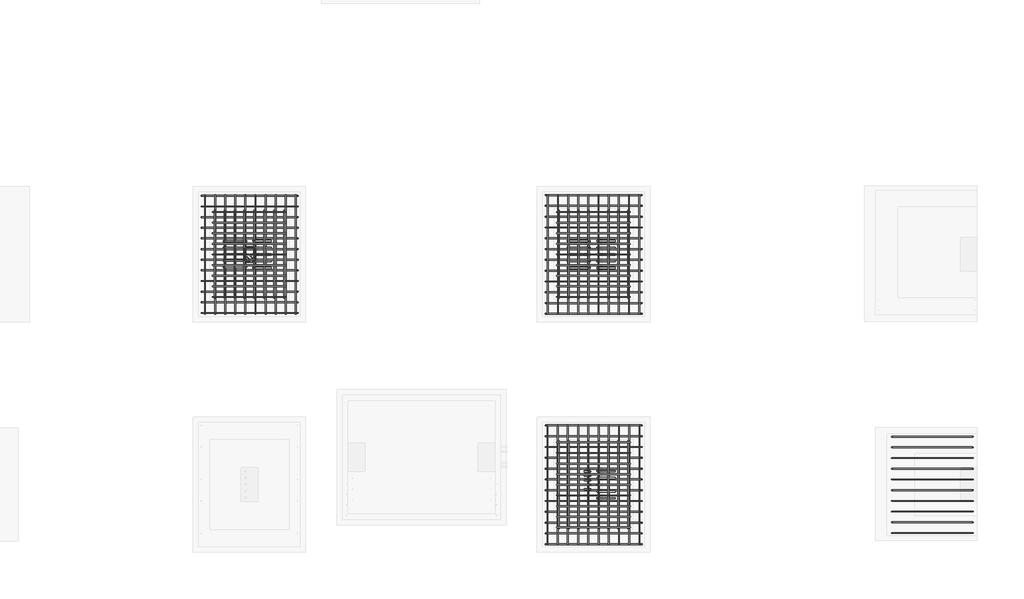
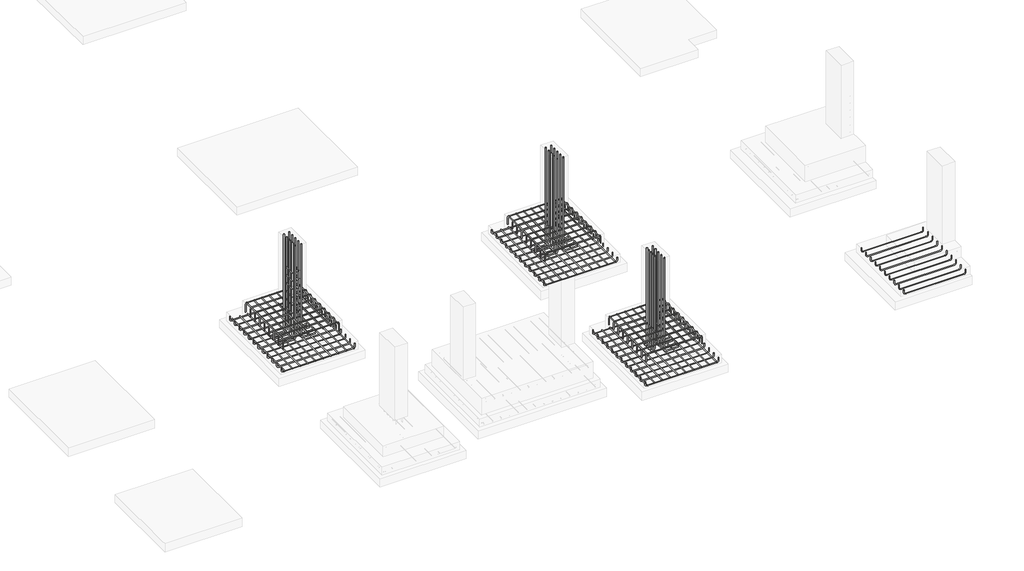
# One storey, part 4 of 6: 20 reinforcing bars.
"""IFC4 building model written with IfcOpenShell, lengths in millimetres."""

from ifc_helpers import new_model, si_unit, point, frame, origin, place, context, project, spatial, polyline, circle_curve, trimmed, segment, composite_curve, source, transform, mapped, element, save
from ifc_brep_helpers import swept_disk

model = new_model("IFC4")

# Units and contexts
model_context = context("Model", 3, world=origin())
ifc_project = project(units=[si_unit("LENGTHUNIT", "METRE", prefix="MILLI")], contexts=[model_context])

# Site, building, storey
site = spatial("IfcSite", under=ifc_project)
building = spatial("IfcBuilding", under=site)
storey = spatial("IfcBuildingStorey", under=building, Elevation=-1828.8)

# Reinforcing bars
placement = place(None, origin())
reinforcing_bar_shape = source(origin(), model_context, "Body", "SolidModel", [
    swept_disk(composite_curve([segment(polyline([(5667706.2007829, -3593857.0523052, -1806.8936208), (5667706.2007829, -3595473.4523052, -1806.8936208)]), True, "CONTINUOUS")], self_intersect=False), 6.0),
])
element("IfcReinforcingBar", 1, at=placement, inside=storey, context=model_context, shape_type="MappedRepresentation", body=[
    mapped(reinforcing_bar_shape, transform((0.0, 0.0, 0.0), x_axis=(1.0, 0.0, 0.0), y_axis=(0.0, 1.0, 0.0), z_axis=(0.0, 0.0, 1.0))),
    mapped(reinforcing_bar_shape, transform((-136.3485017, 0.0, 0.0), x_axis=(1.0, 0.0, 0.0), y_axis=(0.0, 1.0, 0.0), z_axis=(0.0, 0.0, 1.0))),
    mapped(reinforcing_bar_shape, transform((-272.6970034, 0.0, 0.0), x_axis=(1.0, 0.0, 0.0), y_axis=(0.0, 1.0, 0.0), z_axis=(0.0, 0.0, 1.0))),
    mapped(reinforcing_bar_shape, transform((-409.0455051, 0.0, 0.0), x_axis=(1.0, 0.0, 0.0), y_axis=(0.0, 1.0, 0.0), z_axis=(0.0, 0.0, 1.0))),
    mapped(reinforcing_bar_shape, transform((-545.3940068, 0.0, 0.0), x_axis=(1.0, 0.0, 0.0), y_axis=(0.0, 1.0, 0.0), z_axis=(0.0, 0.0, 1.0))),
    mapped(reinforcing_bar_shape, transform((-681.7425085, 0.0, 0.0), x_axis=(1.0, 0.0, 0.0), y_axis=(0.0, 1.0, 0.0), z_axis=(0.0, 0.0, 1.0))),
    mapped(reinforcing_bar_shape, transform((-818.0910101, 0.0, 0.0), x_axis=(1.0, 0.0, 0.0), y_axis=(0.0, 1.0, 0.0), z_axis=(0.0, 0.0, 1.0))),
    mapped(reinforcing_bar_shape, transform((-954.4395118, 0.0, 0.0), x_axis=(1.0, 0.0, 0.0), y_axis=(0.0, 1.0, 0.0), z_axis=(0.0, 0.0, 1.0))),
    mapped(reinforcing_bar_shape, transform((-1090.7880135, 0.0, 0.0), x_axis=(1.0, 0.0, 0.0), y_axis=(0.0, 1.0, 0.0), z_axis=(0.0, 0.0, 1.0))),
    mapped(reinforcing_bar_shape, transform((-1227.1365152, 0.0, 0.0), x_axis=(1.0, 0.0, 0.0), y_axis=(0.0, 1.0, 0.0), z_axis=(0.0, 0.0, 1.0))),
])
reinforcing_bar_2_shape = source(origin(), model_context, "Body", "SolidModel", [
    swept_disk(composite_curve([segment(polyline([(5666582.9165246, -3595238.8523052, -1571.6), (5666582.9165246, -3595238.8523052, -1437.6)]), True, "CONTINUOUS"), segment(trimmed(circle_curve(frame((5666612.9165246, -3595238.8523052, -1437.6), z_axis=(0.0, 1.0, 0.0), x_axis=(-30.0, 0.0, 0.0)), 30.0), [point((5666582.9165246, -3595238.8523052, -1437.6))], [point((5666612.9165246, -3595238.8523052, -1407.6))], True, "CARTESIAN"), True, "CONTINUOUS"), segment(polyline([(5666612.9165246, -3595238.8523052, -1407.6), (5667542.5447698, -3595238.8523052, -1407.6)]), True, "CONTINUOUS"), segment(trimmed(circle_curve(frame((5667542.5447698, -3595238.8523052, -1437.6), z_axis=(0.0, 1.0, 0.0), x_axis=(0.0, 0.0, 30.0)), 30.0), [point((5667542.5447698, -3595238.8523052, -1407.6))], [point((5667572.5447698, -3595238.8523052, -1437.6))], True, "CARTESIAN"), True, "CONTINUOUS"), segment(polyline([(5667572.5447698, -3595238.8523052, -1437.6), (5667572.5447698, -3595238.8523052, -1571.6)]), True, "CONTINUOUS")], self_intersect=False), 6.0),
])
element("IfcReinforcingBar", 2, at=placement, inside=storey, context=model_context, shape_type="MappedRepresentation", body=[
    mapped(reinforcing_bar_2_shape, transform((0.0, 0.0, 0.0), x_axis=(1.0, 0.0, 0.0), y_axis=(0.0, 1.0, 0.0), z_axis=(0.0, 0.0, 1.0))),
    mapped(reinforcing_bar_2_shape, transform((0.0, 143.4, 0.0), x_axis=(1.0, 0.0, 0.0), y_axis=(0.0, 1.0, 0.0), z_axis=(0.0, 0.0, 1.0))),
    mapped(reinforcing_bar_2_shape, transform((0.0, 286.8, 0.0), x_axis=(1.0, 0.0, 0.0), y_axis=(0.0, 1.0, 0.0), z_axis=(0.0, 0.0, 1.0))),
    mapped(reinforcing_bar_2_shape, transform((0.0, 430.2, 0.0), x_axis=(1.0, 0.0, 0.0), y_axis=(0.0, 1.0, 0.0), z_axis=(0.0, 0.0, 1.0))),
    mapped(reinforcing_bar_2_shape, transform((0.0, 573.6, 0.0), x_axis=(1.0, 0.0, 0.0), y_axis=(0.0, 1.0, 0.0), z_axis=(0.0, 0.0, 1.0))),
    mapped(reinforcing_bar_2_shape, transform((0.0, 717.0, 0.0), x_axis=(1.0, 0.0, 0.0), y_axis=(0.0, 1.0, 0.0), z_axis=(0.0, 0.0, 1.0))),
    mapped(reinforcing_bar_2_shape, transform((0.0, 860.4, 0.0), x_axis=(1.0, 0.0, 0.0), y_axis=(0.0, 1.0, 0.0), z_axis=(0.0, 0.0, 1.0))),
    mapped(reinforcing_bar_2_shape, transform((0.0, 1003.8, 0.0), x_axis=(1.0, 0.0, 0.0), y_axis=(0.0, 1.0, 0.0), z_axis=(0.0, 0.0, 1.0))),
    mapped(reinforcing_bar_2_shape, transform((0.0, 1147.2, 0.0), x_axis=(1.0, 0.0, 0.0), y_axis=(0.0, 1.0, 0.0), z_axis=(0.0, 0.0, 1.0))),
])
reinforcing_bar_3_shape = source(origin(), model_context, "Body", "SolidModel", [
    swept_disk(composite_curve([segment(polyline([(5666607.9580652, -3595258.3223129, -1420.5088801), (5666607.9580652, -3594070.7578875, -1420.5088801)]), True, "CONTINUOUS")], self_intersect=False), 6.0),
])
element("IfcReinforcingBar", 3, at=placement, inside=storey, context=model_context, shape_type="MappedRepresentation", body=[
    mapped(reinforcing_bar_3_shape, transform((0.0, 0.0, 0.0), x_axis=(1.0, 0.0, 0.0), y_axis=(0.0, 1.0, 0.0), z_axis=(0.0, 0.0, 1.0))),
    mapped(reinforcing_bar_3_shape, transform((134.2057348, 0.0, 0.0), x_axis=(1.0, 0.0, 0.0), y_axis=(0.0, 1.0, 0.0), z_axis=(0.0, 0.0, 1.0))),
    mapped(reinforcing_bar_3_shape, transform((268.4114695, 0.0, 0.0), x_axis=(1.0, 0.0, 0.0), y_axis=(0.0, 1.0, 0.0), z_axis=(0.0, 0.0, 1.0))),
    mapped(reinforcing_bar_3_shape, transform((402.6172043, 0.0, 0.0), x_axis=(1.0, 0.0, 0.0), y_axis=(0.0, 1.0, 0.0), z_axis=(0.0, 0.0, 1.0))),
    mapped(reinforcing_bar_3_shape, transform((536.8229391, 0.0, 0.0), x_axis=(1.0, 0.0, 0.0), y_axis=(0.0, 1.0, 0.0), z_axis=(0.0, 0.0, 1.0))),
    mapped(reinforcing_bar_3_shape, transform((671.0286738, 0.0, 0.0), x_axis=(1.0, 0.0, 0.0), y_axis=(0.0, 1.0, 0.0), z_axis=(0.0, 0.0, 1.0))),
    mapped(reinforcing_bar_3_shape, transform((805.2344086, 0.0, 0.0), x_axis=(1.0, 0.0, 0.0), y_axis=(0.0, 1.0, 0.0), z_axis=(0.0, 0.0, 1.0))),
    mapped(reinforcing_bar_3_shape, transform((939.4401433, 0.0, 0.0), x_axis=(1.0, 0.0, 0.0), y_axis=(0.0, 1.0, 0.0), z_axis=(0.0, 0.0, 1.0))),
])
reinforcing_bar_4_shape = source(origin(), model_context, "Body", "SolidModel", [
    swept_disk(composite_curve([segment(polyline([(5672341.0341193, -3593857.0523052, -1804.5123708), (5672341.0341193, -3595473.4523052, -1804.5123708)]), True, "CONTINUOUS")], self_intersect=False), 6.0),
])
element("IfcReinforcingBar", 4, at=placement, inside=storey, context=model_context, shape_type="MappedRepresentation", body=[
    mapped(reinforcing_bar_4_shape, transform((0.0, 0.0, 0.0), x_axis=(1.0, 0.0, 0.0), y_axis=(0.0, 1.0, 0.0), z_axis=(0.0, 0.0, 1.0))),
    mapped(reinforcing_bar_4_shape, transform((-136.9779353, 0.0, 0.0), x_axis=(1.0, 0.0, 0.0), y_axis=(0.0, 1.0, 0.0), z_axis=(0.0, 0.0, 1.0))),
    mapped(reinforcing_bar_4_shape, transform((-273.9558706, 0.0, 0.0), x_axis=(1.0, 0.0, 0.0), y_axis=(0.0, 1.0, 0.0), z_axis=(0.0, 0.0, 1.0))),
    mapped(reinforcing_bar_4_shape, transform((-410.9338059, 0.0, 0.0), x_axis=(1.0, 0.0, 0.0), y_axis=(0.0, 1.0, 0.0), z_axis=(0.0, 0.0, 1.0))),
    mapped(reinforcing_bar_4_shape, transform((-547.9117413, 0.0, 0.0), x_axis=(1.0, 0.0, 0.0), y_axis=(0.0, 1.0, 0.0), z_axis=(0.0, 0.0, 1.0))),
    mapped(reinforcing_bar_4_shape, transform((-684.8896766, 0.0, 0.0), x_axis=(1.0, 0.0, 0.0), y_axis=(0.0, 1.0, 0.0), z_axis=(0.0, 0.0, 1.0))),
    mapped(reinforcing_bar_4_shape, transform((-821.8676119, 0.0, 0.0), x_axis=(1.0, 0.0, 0.0), y_axis=(0.0, 1.0, 0.0), z_axis=(0.0, 0.0, 1.0))),
    mapped(reinforcing_bar_4_shape, transform((-958.8455472, 0.0, 0.0), x_axis=(1.0, 0.0, 0.0), y_axis=(0.0, 1.0, 0.0), z_axis=(0.0, 0.0, 1.0))),
    mapped(reinforcing_bar_4_shape, transform((-1095.8234825, 0.0, 0.0), x_axis=(1.0, 0.0, 0.0), y_axis=(0.0, 1.0, 0.0), z_axis=(0.0, 0.0, 1.0))),
    mapped(reinforcing_bar_4_shape, transform((-1232.8014178, 0.0, 0.0), x_axis=(1.0, 0.0, 0.0), y_axis=(0.0, 1.0, 0.0), z_axis=(0.0, 0.0, 1.0))),
])
reinforcing_bar_5_shape = source(origin(), model_context, "Body", "SolidModel", [
    swept_disk(composite_curve([segment(polyline([(5671231.1165246, -3595238.8523052, -1551.6), (5671231.1165246, -3595238.8523052, -1437.6)]), True, "CONTINUOUS"), segment(trimmed(circle_curve(frame((5671261.1165246, -3595238.8523052, -1437.6), z_axis=(0.0, 1.0, 0.0), x_axis=(-30.0, 0.0, 0.0)), 30.0), [point((5671231.1165246, -3595238.8523052, -1437.6))], [point((5671261.1165246, -3595238.8523052, -1407.6))], True, "CARTESIAN"), True, "CONTINUOUS"), segment(polyline([(5671261.1165246, -3595238.8523052, -1407.6), (5672186.288821, -3595238.8523052, -1407.6)]), True, "CONTINUOUS"), segment(trimmed(circle_curve(frame((5672186.288821, -3595238.8523052, -1437.6), z_axis=(0.0, 1.0, 0.0), x_axis=(0.0, 0.0, 30.0)), 30.0), [point((5672186.288821, -3595238.8523052, -1407.6))], [point((5672216.288821, -3595238.8523052, -1437.6))], True, "CARTESIAN"), True, "CONTINUOUS"), segment(polyline([(5672216.288821, -3595238.8523052, -1437.6), (5672216.288821, -3595238.8523052, -1551.6)]), True, "CONTINUOUS")], self_intersect=False), 6.0),
])
element("IfcReinforcingBar", 5, at=placement, inside=storey, context=model_context, shape_type="MappedRepresentation", body=[
    mapped(reinforcing_bar_5_shape, transform((0.0, 0.0, 0.0), x_axis=(1.0, 0.0, 0.0), y_axis=(0.0, 1.0, 0.0), z_axis=(0.0, 0.0, 1.0))),
    mapped(reinforcing_bar_5_shape, transform((0.0, 143.4, 0.0), x_axis=(1.0, 0.0, 0.0), y_axis=(0.0, 1.0, 0.0), z_axis=(0.0, 0.0, 1.0))),
    mapped(reinforcing_bar_5_shape, transform((0.0, 286.8, 0.0), x_axis=(1.0, 0.0, 0.0), y_axis=(0.0, 1.0, 0.0), z_axis=(0.0, 0.0, 1.0))),
    mapped(reinforcing_bar_5_shape, transform((0.0, 430.2, 0.0), x_axis=(1.0, 0.0, 0.0), y_axis=(0.0, 1.0, 0.0), z_axis=(0.0, 0.0, 1.0))),
    mapped(reinforcing_bar_5_shape, transform((0.0, 573.6, 0.0), x_axis=(1.0, 0.0, 0.0), y_axis=(0.0, 1.0, 0.0), z_axis=(0.0, 0.0, 1.0))),
    mapped(reinforcing_bar_5_shape, transform((0.0, 717.0, 0.0), x_axis=(1.0, 0.0, 0.0), y_axis=(0.0, 1.0, 0.0), z_axis=(0.0, 0.0, 1.0))),
    mapped(reinforcing_bar_5_shape, transform((0.0, 860.4, 0.0), x_axis=(1.0, 0.0, 0.0), y_axis=(0.0, 1.0, 0.0), z_axis=(0.0, 0.0, 1.0))),
    mapped(reinforcing_bar_5_shape, transform((0.0, 1003.8, 0.0), x_axis=(1.0, 0.0, 0.0), y_axis=(0.0, 1.0, 0.0), z_axis=(0.0, 0.0, 1.0))),
    mapped(reinforcing_bar_5_shape, transform((0.0, 1147.2, 0.0), x_axis=(1.0, 0.0, 0.0), y_axis=(0.0, 1.0, 0.0), z_axis=(0.0, 0.0, 1.0))),
])
reinforcing_bar_6_shape = source(origin(), model_context, "Body", "SolidModel", [
    swept_disk(composite_curve([segment(polyline([(5671259.1917143, -3595258.3223129, -1419.7151301), (5671259.1917143, -3594070.7578875, -1419.7151301)]), True, "CONTINUOUS")], self_intersect=False), 6.0),
])
element("IfcReinforcingBar", 6, at=placement, inside=storey, context=model_context, shape_type="MappedRepresentation", body=[
    mapped(reinforcing_bar_6_shape, transform((0.0, 0.0, 0.0), x_axis=(1.0, 0.0, 0.0), y_axis=(0.0, 1.0, 0.0), z_axis=(0.0, 0.0, 1.0))),
    mapped(reinforcing_bar_6_shape, transform((133.142035, 0.0, 0.0), x_axis=(1.0, 0.0, 0.0), y_axis=(0.0, 1.0, 0.0), z_axis=(0.0, 0.0, 1.0))),
    mapped(reinforcing_bar_6_shape, transform((266.28407, 0.0, 0.0), x_axis=(1.0, 0.0, 0.0), y_axis=(0.0, 1.0, 0.0), z_axis=(0.0, 0.0, 1.0))),
    mapped(reinforcing_bar_6_shape, transform((399.426105, 0.0, 0.0), x_axis=(1.0, 0.0, 0.0), y_axis=(0.0, 1.0, 0.0), z_axis=(0.0, 0.0, 1.0))),
    mapped(reinforcing_bar_6_shape, transform((532.56814, 0.0, 0.0), x_axis=(1.0, 0.0, 0.0), y_axis=(0.0, 1.0, 0.0), z_axis=(0.0, 0.0, 1.0))),
    mapped(reinforcing_bar_6_shape, transform((665.7101749, 0.0, 0.0), x_axis=(1.0, 0.0, 0.0), y_axis=(0.0, 1.0, 0.0), z_axis=(0.0, 0.0, 1.0))),
    mapped(reinforcing_bar_6_shape, transform((798.8522099, 0.0, 0.0), x_axis=(1.0, 0.0, 0.0), y_axis=(0.0, 1.0, 0.0), z_axis=(0.0, 0.0, 1.0))),
    mapped(reinforcing_bar_6_shape, transform((931.9942449, 0.0, 0.0), x_axis=(1.0, 0.0, 0.0), y_axis=(0.0, 1.0, 0.0), z_axis=(0.0, 0.0, 1.0))),
])
reinforcing_bar_7_shape = source(origin(), model_context, "Body", "SolidModel", [
    swept_disk(composite_curve([segment(polyline([(5672346.3995476, -3596967.8875145, -1801.3373708), (5672346.3995476, -3598584.2875145, -1801.3373708)]), True, "CONTINUOUS")], self_intersect=False), 6.0),
])
element("IfcReinforcingBar", 7, at=placement, inside=storey, context=model_context, shape_type="MappedRepresentation", body=[
    mapped(reinforcing_bar_7_shape, transform((0.0, 0.0, 0.0), x_axis=(1.0, 0.0, 0.0), y_axis=(0.0, 1.0, 0.0), z_axis=(0.0, 0.0, 1.0))),
    mapped(reinforcing_bar_7_shape, transform((-138.145428, 0.0, 0.0), x_axis=(1.0, 0.0, 0.0), y_axis=(0.0, 1.0, 0.0), z_axis=(0.0, 0.0, 1.0))),
    mapped(reinforcing_bar_7_shape, transform((-276.2908559, 0.0, 0.0), x_axis=(1.0, 0.0, 0.0), y_axis=(0.0, 1.0, 0.0), z_axis=(0.0, 0.0, 1.0))),
    mapped(reinforcing_bar_7_shape, transform((-414.4362839, 0.0, 0.0), x_axis=(1.0, 0.0, 0.0), y_axis=(0.0, 1.0, 0.0), z_axis=(0.0, 0.0, 1.0))),
    mapped(reinforcing_bar_7_shape, transform((-552.5817118, 0.0, 0.0), x_axis=(1.0, 0.0, 0.0), y_axis=(0.0, 1.0, 0.0), z_axis=(0.0, 0.0, 1.0))),
    mapped(reinforcing_bar_7_shape, transform((-690.7271398, 0.0, 0.0), x_axis=(1.0, 0.0, 0.0), y_axis=(0.0, 1.0, 0.0), z_axis=(0.0, 0.0, 1.0))),
    mapped(reinforcing_bar_7_shape, transform((-828.8725677, 0.0, 0.0), x_axis=(1.0, 0.0, 0.0), y_axis=(0.0, 1.0, 0.0), z_axis=(0.0, 0.0, 1.0))),
    mapped(reinforcing_bar_7_shape, transform((-967.0179957, 0.0, 0.0), x_axis=(1.0, 0.0, 0.0), y_axis=(0.0, 1.0, 0.0), z_axis=(0.0, 0.0, 1.0))),
    mapped(reinforcing_bar_7_shape, transform((-1105.1634236, 0.0, 0.0), x_axis=(1.0, 0.0, 0.0), y_axis=(0.0, 1.0, 0.0), z_axis=(0.0, 0.0, 1.0))),
    mapped(reinforcing_bar_7_shape, transform((-1243.3088516, 0.0, 0.0), x_axis=(1.0, 0.0, 0.0), y_axis=(0.0, 1.0, 0.0), z_axis=(0.0, 0.0, 1.0))),
])
reinforcing_bar_8_shape = source(origin(), model_context, "Body", "SolidModel", [
    swept_disk(composite_curve([segment(polyline([(5671231.1165246, -3598349.6875145, -1551.6), (5671231.1165246, -3598349.6875145, -1437.6)]), True, "CONTINUOUS"), segment(trimmed(circle_curve(frame((5671261.1165246, -3598349.6875145, -1437.6), z_axis=(0.0, 1.0, 0.0), x_axis=(-30.0, 0.0, 0.0)), 30.0), [point((5671231.1165246, -3598349.6875145, -1437.6))], [point((5671261.1165246, -3598349.6875145, -1407.6))], True, "CARTESIAN"), True, "CONTINUOUS"), segment(polyline([(5671261.1165246, -3598349.6875145, -1407.6), (5672189.8759026, -3598349.6875145, -1407.6)]), True, "CONTINUOUS"), segment(trimmed(circle_curve(frame((5672189.8759026, -3598349.6875145, -1437.6), z_axis=(0.0, 1.0, 0.0), x_axis=(0.0, 0.0, 30.0)), 30.0), [point((5672189.8759026, -3598349.6875145, -1407.6))], [point((5672219.8759026, -3598349.6875145, -1437.6))], True, "CARTESIAN"), True, "CONTINUOUS"), segment(polyline([(5672219.8759026, -3598349.6875145, -1437.6), (5672219.8759026, -3598349.6875145, -1551.6)]), True, "CONTINUOUS")], self_intersect=False), 6.0),
])
element("IfcReinforcingBar", 8, at=placement, inside=storey, context=model_context, shape_type="MappedRepresentation", body=[
    mapped(reinforcing_bar_8_shape, transform((0.0, 0.0, 0.0), x_axis=(1.0, 0.0, 0.0), y_axis=(0.0, 1.0, 0.0), z_axis=(0.0, 0.0, 1.0))),
    mapped(reinforcing_bar_8_shape, transform((0.0, 143.4, 0.0), x_axis=(1.0, 0.0, 0.0), y_axis=(0.0, 1.0, 0.0), z_axis=(0.0, 0.0, 1.0))),
    mapped(reinforcing_bar_8_shape, transform((0.0, 286.8, 0.0), x_axis=(1.0, 0.0, 0.0), y_axis=(0.0, 1.0, 0.0), z_axis=(0.0, 0.0, 1.0))),
    mapped(reinforcing_bar_8_shape, transform((0.0, 430.2, 0.0), x_axis=(1.0, 0.0, 0.0), y_axis=(0.0, 1.0, 0.0), z_axis=(0.0, 0.0, 1.0))),
    mapped(reinforcing_bar_8_shape, transform((0.0, 573.6, 0.0), x_axis=(1.0, 0.0, 0.0), y_axis=(0.0, 1.0, 0.0), z_axis=(0.0, 0.0, 1.0))),
    mapped(reinforcing_bar_8_shape, transform((0.0, 717.0, 0.0), x_axis=(1.0, 0.0, 0.0), y_axis=(0.0, 1.0, 0.0), z_axis=(0.0, 0.0, 1.0))),
    mapped(reinforcing_bar_8_shape, transform((0.0, 860.4, 0.0), x_axis=(1.0, 0.0, 0.0), y_axis=(0.0, 1.0, 0.0), z_axis=(0.0, 0.0, 1.0))),
    mapped(reinforcing_bar_8_shape, transform((0.0, 1003.8, 0.0), x_axis=(1.0, 0.0, 0.0), y_axis=(0.0, 1.0, 0.0), z_axis=(0.0, 0.0, 1.0))),
    mapped(reinforcing_bar_8_shape, transform((0.0, 1147.2, 0.0), x_axis=(1.0, 0.0, 0.0), y_axis=(0.0, 1.0, 0.0), z_axis=(0.0, 0.0, 1.0))),
])
reinforcing_bar_9_shape = source(origin(), model_context, "Body", "SolidModel", [
    swept_disk(composite_curve([segment(polyline([(5671255.1855198, -3598369.1575222, -1420.5088801), (5671255.1855198, -3597181.5930968, -1420.5088801)]), True, "CONTINUOUS")], self_intersect=False), 6.0),
])
element("IfcReinforcingBar", 9, at=placement, inside=storey, context=model_context, shape_type="MappedRepresentation", body=[
    mapped(reinforcing_bar_9_shape, transform((0.0, 0.0, 0.0), x_axis=(1.0, 0.0, 0.0), y_axis=(0.0, 1.0, 0.0), z_axis=(0.0, 0.0, 1.0))),
    mapped(reinforcing_bar_9_shape, transform((134.2050832, 0.0, 0.0), x_axis=(1.0, 0.0, 0.0), y_axis=(0.0, 1.0, 0.0), z_axis=(0.0, 0.0, 1.0))),
    mapped(reinforcing_bar_9_shape, transform((268.4101664, 0.0, 0.0), x_axis=(1.0, 0.0, 0.0), y_axis=(0.0, 1.0, 0.0), z_axis=(0.0, 0.0, 1.0))),
    mapped(reinforcing_bar_9_shape, transform((402.6152497, 0.0, 0.0), x_axis=(1.0, 0.0, 0.0), y_axis=(0.0, 1.0, 0.0), z_axis=(0.0, 0.0, 1.0))),
    mapped(reinforcing_bar_9_shape, transform((536.8203329, 0.0, 0.0), x_axis=(1.0, 0.0, 0.0), y_axis=(0.0, 1.0, 0.0), z_axis=(0.0, 0.0, 1.0))),
    mapped(reinforcing_bar_9_shape, transform((671.0254161, 0.0, 0.0), x_axis=(1.0, 0.0, 0.0), y_axis=(0.0, 1.0, 0.0), z_axis=(0.0, 0.0, 1.0))),
    mapped(reinforcing_bar_9_shape, transform((805.2304993, 0.0, 0.0), x_axis=(1.0, 0.0, 0.0), y_axis=(0.0, 1.0, 0.0), z_axis=(0.0, 0.0, 1.0))),
    mapped(reinforcing_bar_9_shape, transform((939.4355826, 0.0, 0.0), x_axis=(1.0, 0.0, 0.0), y_axis=(0.0, 1.0, 0.0), z_axis=(0.0, 0.0, 1.0))),
])
reinforcing_bar_10_shape = source(origin(), model_context, "Body", "SolidModel", [
    swept_disk(composite_curve([segment(polyline([(5666430.5165246, -3593873.2144717, -1739.9194349), (5666430.5165246, -3593873.2144717, -1788.9194349)]), True, "CONTINUOUS"), segment(trimmed(circle_curve(frame((5666460.5165246, -3593873.2144717, -1788.9194349), z_axis=(0.0, -1.0, 0.0), x_axis=(-30.0, 0.0, 0.0)), 30.0), [point((5666430.5165246, -3593873.2144717, -1788.9194349))], [point((5666460.5165246, -3593873.2144717, -1818.9194349))], True, "CARTESIAN"), True, "CONTINUOUS"), segment(polyline([(5666460.5165246, -3593873.2144717, -1818.9194349), (5667700.1165246, -3593873.2144717, -1818.9194349)]), True, "CONTINUOUS"), segment(trimmed(circle_curve(frame((5667700.1165246, -3593873.2144717, -1788.9194349), z_axis=(0.0, -1.0, 0.0), x_axis=(0.0, 0.0, -30.0)), 30.0), [point((5667700.1165246, -3593873.2144717, -1818.9194349))], [point((5667730.1165246, -3593873.2144717, -1788.9194349))], True, "CARTESIAN"), True, "CONTINUOUS"), segment(polyline([(5667730.1165246, -3593873.2144717, -1788.9194349), (5667730.1165246, -3593873.2144717, -1739.9194349)]), True, "CONTINUOUS")], self_intersect=False), 6.0),
])
element("IfcReinforcingBar", 10, at=placement, inside=storey, context=model_context, shape_type="MappedRepresentation", body=[
    mapped(reinforcing_bar_10_shape, transform((0.0, 0.0, 0.0), x_axis=(1.0, 0.0, 0.0), y_axis=(0.0, 1.0, 0.0), z_axis=(0.0, 0.0, 1.0))),
    mapped(reinforcing_bar_10_shape, transform((0.0, -143.7721492, 0.0), x_axis=(1.0, 0.0, 0.0), y_axis=(0.0, 1.0, 0.0), z_axis=(0.0, 0.0, 1.0))),
    mapped(reinforcing_bar_10_shape, transform((0.0, -287.5442983, 0.0), x_axis=(1.0, 0.0, 0.0), y_axis=(0.0, 1.0, 0.0), z_axis=(0.0, 0.0, 1.0))),
    mapped(reinforcing_bar_10_shape, transform((0.0, -431.3164475, 0.0), x_axis=(1.0, 0.0, 0.0), y_axis=(0.0, 1.0, 0.0), z_axis=(0.0, 0.0, 1.0))),
    mapped(reinforcing_bar_10_shape, transform((0.0, -575.0885967, 0.0), x_axis=(1.0, 0.0, 0.0), y_axis=(0.0, 1.0, 0.0), z_axis=(0.0, 0.0, 1.0))),
    mapped(reinforcing_bar_10_shape, transform((0.0, -718.8607458, 0.0), x_axis=(1.0, 0.0, 0.0), y_axis=(0.0, 1.0, 0.0), z_axis=(0.0, 0.0, 1.0))),
    mapped(reinforcing_bar_10_shape, transform((0.0, -862.632895, 0.0), x_axis=(1.0, 0.0, 0.0), y_axis=(0.0, 1.0, 0.0), z_axis=(0.0, 0.0, 1.0))),
    mapped(reinforcing_bar_10_shape, transform((0.0, -1006.4050441, 0.0), x_axis=(1.0, 0.0, 0.0), y_axis=(0.0, 1.0, 0.0), z_axis=(0.0, 0.0, 1.0))),
    mapped(reinforcing_bar_10_shape, transform((0.0, -1150.1771933, 0.0), x_axis=(1.0, 0.0, 0.0), y_axis=(0.0, 1.0, 0.0), z_axis=(0.0, 0.0, 1.0))),
    mapped(reinforcing_bar_10_shape, transform((0.0, -1293.9493425, 0.0), x_axis=(1.0, 0.0, 0.0), y_axis=(0.0, 1.0, 0.0), z_axis=(0.0, 0.0, 1.0))),
    mapped(reinforcing_bar_10_shape, transform((0.0, -1437.7214916, 0.0), x_axis=(1.0, 0.0, 0.0), y_axis=(0.0, 1.0, 0.0), z_axis=(0.0, 0.0, 1.0))),
    mapped(reinforcing_bar_10_shape, transform((0.0, -1581.4936408, 0.0), x_axis=(1.0, 0.0, 0.0), y_axis=(0.0, 1.0, 0.0), z_axis=(0.0, 0.0, 1.0))),
])
reinforcing_bar_11_shape = source(origin(), model_context, "Body", "SolidModel", [
    swept_disk(composite_curve([segment(polyline([(5675753.0030838, -3597125.2875145, -1738.4709043), (5675753.0030838, -3597125.2875145, -1793.4709043)]), True, "CONTINUOUS"), segment(trimmed(circle_curve(frame((5675778.0030838, -3597125.2875145, -1793.4709043), z_axis=(0.0, -1.0, 0.0), x_axis=(-25.0, 0.0, 0.0)), 25.0), [point((5675753.0030838, -3597125.2875145, -1793.4709043))], [point((5675778.0030838, -3597125.2875145, -1818.4709043))], True, "CARTESIAN"), True, "CONTINUOUS"), segment(polyline([(5675778.0030838, -3597125.2875145, -1818.4709043), (5676824.5916392, -3597125.2875145, -1818.4709043)]), True, "CONTINUOUS"), segment(trimmed(circle_curve(frame((5676824.5916392, -3597125.2875145, -1793.4709043), z_axis=(0.0, -1.0, 0.0), x_axis=(0.0, 0.0, -25.0)), 25.0), [point((5676824.5916392, -3597125.2875145, -1818.4709043))], [point((5676849.5916392, -3597125.2875145, -1793.4709043))], True, "CARTESIAN"), True, "CONTINUOUS"), segment(polyline([(5676849.5916392, -3597125.2875145, -1793.4709043), (5676849.5916392, -3597125.2875145, -1738.4709043)]), True, "CONTINUOUS")], self_intersect=False), 5.0),
])
element("IfcReinforcingBar", 11, at=placement, inside=storey, context=model_context, shape_type="MappedRepresentation", body=[
    mapped(reinforcing_bar_11_shape, transform((0.0, 0.0, 0.0), x_axis=(1.0, 0.0, 0.0), y_axis=(0.0, 1.0, 0.0), z_axis=(0.0, 0.0, 1.0))),
    mapped(reinforcing_bar_11_shape, transform((0.0, -144.6222222, 0.0), x_axis=(1.0, 0.0, 0.0), y_axis=(0.0, 1.0, 0.0), z_axis=(0.0, 0.0, 1.0))),
    mapped(reinforcing_bar_11_shape, transform((0.0, -289.2444444, 0.0), x_axis=(1.0, 0.0, 0.0), y_axis=(0.0, 1.0, 0.0), z_axis=(0.0, 0.0, 1.0))),
    mapped(reinforcing_bar_11_shape, transform((0.0, -433.8666667, 0.0), x_axis=(1.0, 0.0, 0.0), y_axis=(0.0, 1.0, 0.0), z_axis=(0.0, 0.0, 1.0))),
    mapped(reinforcing_bar_11_shape, transform((0.0, -578.4888889, 0.0), x_axis=(1.0, 0.0, 0.0), y_axis=(0.0, 1.0, 0.0), z_axis=(0.0, 0.0, 1.0))),
    mapped(reinforcing_bar_11_shape, transform((0.0, -723.1111111, 0.0), x_axis=(1.0, 0.0, 0.0), y_axis=(0.0, 1.0, 0.0), z_axis=(0.0, 0.0, 1.0))),
    mapped(reinforcing_bar_11_shape, transform((0.0, -867.7333333, 0.0), x_axis=(1.0, 0.0, 0.0), y_axis=(0.0, 1.0, 0.0), z_axis=(0.0, 0.0, 1.0))),
    mapped(reinforcing_bar_11_shape, transform((0.0, -1012.3555556, 0.0), x_axis=(1.0, 0.0, 0.0), y_axis=(0.0, 1.0, 0.0), z_axis=(0.0, 0.0, 1.0))),
    mapped(reinforcing_bar_11_shape, transform((0.0, -1156.9777778, 0.0), x_axis=(1.0, 0.0, 0.0), y_axis=(0.0, 1.0, 0.0), z_axis=(0.0, 0.0, 1.0))),
    mapped(reinforcing_bar_11_shape, transform((0.0, -1301.6, 0.0), x_axis=(1.0, 0.0, 0.0), y_axis=(0.0, 1.0, 0.0), z_axis=(0.0, 0.0, 1.0))),
])
reinforcing_bar_12_shape = source(origin(), model_context, "Body", "SolidModel", [
    swept_disk(composite_curve([segment(polyline([(5671078.7165246, -3593863.0523052, -1743.8), (5671078.7165246, -3593863.0523052, -1787.0006094)]), True, "CONTINUOUS"), segment(trimmed(circle_curve(frame((5671108.7165246, -3593863.0523052, -1787.0006094), z_axis=(0.0, -1.0, 0.0), x_axis=(-30.0, 0.0, 0.0)), 30.0), [point((5671078.7165246, -3593863.0523052, -1787.0006094))], [point((5671108.7165246, -3593863.0523052, -1817.0006094))], True, "CARTESIAN"), True, "CONTINUOUS"), segment(polyline([(5671108.7165246, -3593863.0523052, -1817.0006094), (5672348.3165246, -3593863.0523052, -1817.0006094)]), True, "CONTINUOUS"), segment(trimmed(circle_curve(frame((5672348.3165246, -3593863.0523052, -1787.0006094), z_axis=(0.0, -1.0, 0.0), x_axis=(0.0, 0.0, -30.0)), 30.0), [point((5672348.3165246, -3593863.0523052, -1817.0006094))], [point((5672378.3165246, -3593863.0523052, -1787.0006094))], True, "CARTESIAN"), True, "CONTINUOUS"), segment(polyline([(5672378.3165246, -3593863.0523052, -1787.0006094), (5672378.3165246, -3593863.0523052, -1743.8)]), True, "CONTINUOUS")], self_intersect=False), 6.0),
])
element("IfcReinforcingBar", 12, at=placement, inside=storey, context=model_context, shape_type="MappedRepresentation", body=[
    mapped(reinforcing_bar_12_shape, transform((0.0, 0.0, 0.0), x_axis=(1.0, 0.0, 0.0), y_axis=(0.0, 1.0, 0.0), z_axis=(0.0, 0.0, 1.0))),
    mapped(reinforcing_bar_12_shape, transform((0.0, -145.8545455, 0.0), x_axis=(1.0, 0.0, 0.0), y_axis=(0.0, 1.0, 0.0), z_axis=(0.0, 0.0, 1.0))),
    mapped(reinforcing_bar_12_shape, transform((0.0, -291.7090909, 0.0), x_axis=(1.0, 0.0, 0.0), y_axis=(0.0, 1.0, 0.0), z_axis=(0.0, 0.0, 1.0))),
    mapped(reinforcing_bar_12_shape, transform((0.0, -437.5636364, 0.0), x_axis=(1.0, 0.0, 0.0), y_axis=(0.0, 1.0, 0.0), z_axis=(0.0, 0.0, 1.0))),
    mapped(reinforcing_bar_12_shape, transform((0.0, -583.4181818, 0.0), x_axis=(1.0, 0.0, 0.0), y_axis=(0.0, 1.0, 0.0), z_axis=(0.0, 0.0, 1.0))),
    mapped(reinforcing_bar_12_shape, transform((0.0, -729.2727273, 0.0), x_axis=(1.0, 0.0, 0.0), y_axis=(0.0, 1.0, 0.0), z_axis=(0.0, 0.0, 1.0))),
    mapped(reinforcing_bar_12_shape, transform((0.0, -875.1272727, 0.0), x_axis=(1.0, 0.0, 0.0), y_axis=(0.0, 1.0, 0.0), z_axis=(0.0, 0.0, 1.0))),
    mapped(reinforcing_bar_12_shape, transform((0.0, -1020.9818182, 0.0), x_axis=(1.0, 0.0, 0.0), y_axis=(0.0, 1.0, 0.0), z_axis=(0.0, 0.0, 1.0))),
    mapped(reinforcing_bar_12_shape, transform((0.0, -1166.8363636, 0.0), x_axis=(1.0, 0.0, 0.0), y_axis=(0.0, 1.0, 0.0), z_axis=(0.0, 0.0, 1.0))),
    mapped(reinforcing_bar_12_shape, transform((0.0, -1312.6909091, 0.0), x_axis=(1.0, 0.0, 0.0), y_axis=(0.0, 1.0, 0.0), z_axis=(0.0, 0.0, 1.0))),
    mapped(reinforcing_bar_12_shape, transform((0.0, -1458.5454545, 0.0), x_axis=(1.0, 0.0, 0.0), y_axis=(0.0, 1.0, 0.0), z_axis=(0.0, 0.0, 1.0))),
    mapped(reinforcing_bar_12_shape, transform((0.0, -1604.4, 0.0), x_axis=(1.0, 0.0, 0.0), y_axis=(0.0, 1.0, 0.0), z_axis=(0.0, 0.0, 1.0))),
])
reinforcing_bar_13_shape = source(origin(), model_context, "Body", "SolidModel", [
    swept_disk(composite_curve([segment(polyline([(5671078.7165246, -3596973.8875145, -1735.2729024), (5671078.7165246, -3596973.8875145, -1784.2729024)]), True, "CONTINUOUS"), segment(trimmed(circle_curve(frame((5671108.7165246, -3596973.8875145, -1784.2729024), z_axis=(0.0, -1.0, 0.0), x_axis=(-30.0, 0.0, 0.0)), 30.0), [point((5671078.7165246, -3596973.8875145, -1784.2729024))], [point((5671108.7165246, -3596973.8875145, -1814.2729024))], True, "CARTESIAN"), True, "CONTINUOUS"), segment(polyline([(5671108.7165246, -3596973.8875145, -1814.2729024), (5672348.3165246, -3596973.8875145, -1814.2729024)]), True, "CONTINUOUS"), segment(trimmed(circle_curve(frame((5672348.3165246, -3596973.8875145, -1784.2729024), z_axis=(0.0, -1.0, 0.0), x_axis=(0.0, 0.0, -30.0)), 30.0), [point((5672348.3165246, -3596973.8875145, -1814.2729024))], [point((5672378.3165246, -3596973.8875145, -1784.2729024))], True, "CARTESIAN"), True, "CONTINUOUS"), segment(polyline([(5672378.3165246, -3596973.8875145, -1784.2729024), (5672378.3165246, -3596973.8875145, -1735.2729024)]), True, "CONTINUOUS")], self_intersect=False), 6.0),
])
element("IfcReinforcingBar", 13, at=placement, inside=storey, context=model_context, shape_type="MappedRepresentation", body=[
    mapped(reinforcing_bar_13_shape, transform((0.0, 0.0, 0.0), x_axis=(1.0, 0.0, 0.0), y_axis=(0.0, 1.0, 0.0), z_axis=(0.0, 0.0, 1.0))),
    mapped(reinforcing_bar_13_shape, transform((0.0, -145.8545455, 0.0), x_axis=(1.0, 0.0, 0.0), y_axis=(0.0, 1.0, 0.0), z_axis=(0.0, 0.0, 1.0))),
    mapped(reinforcing_bar_13_shape, transform((0.0, -291.7090909, 0.0), x_axis=(1.0, 0.0, 0.0), y_axis=(0.0, 1.0, 0.0), z_axis=(0.0, 0.0, 1.0))),
    mapped(reinforcing_bar_13_shape, transform((0.0, -437.5636364, 0.0), x_axis=(1.0, 0.0, 0.0), y_axis=(0.0, 1.0, 0.0), z_axis=(0.0, 0.0, 1.0))),
    mapped(reinforcing_bar_13_shape, transform((0.0, -583.4181818, 0.0), x_axis=(1.0, 0.0, 0.0), y_axis=(0.0, 1.0, 0.0), z_axis=(0.0, 0.0, 1.0))),
    mapped(reinforcing_bar_13_shape, transform((0.0, -729.2727273, 0.0), x_axis=(1.0, 0.0, 0.0), y_axis=(0.0, 1.0, 0.0), z_axis=(0.0, 0.0, 1.0))),
    mapped(reinforcing_bar_13_shape, transform((0.0, -875.1272727, 0.0), x_axis=(1.0, 0.0, 0.0), y_axis=(0.0, 1.0, 0.0), z_axis=(0.0, 0.0, 1.0))),
    mapped(reinforcing_bar_13_shape, transform((0.0, -1020.9818182, 0.0), x_axis=(1.0, 0.0, 0.0), y_axis=(0.0, 1.0, 0.0), z_axis=(0.0, 0.0, 1.0))),
    mapped(reinforcing_bar_13_shape, transform((0.0, -1166.8363636, 0.0), x_axis=(1.0, 0.0, 0.0), y_axis=(0.0, 1.0, 0.0), z_axis=(0.0, 0.0, 1.0))),
    mapped(reinforcing_bar_13_shape, transform((0.0, -1312.6909091, 0.0), x_axis=(1.0, 0.0, 0.0), y_axis=(0.0, 1.0, 0.0), z_axis=(0.0, 0.0, 1.0))),
    mapped(reinforcing_bar_13_shape, transform((0.0, -1458.5454545, 0.0), x_axis=(1.0, 0.0, 0.0), y_axis=(0.0, 1.0, 0.0), z_axis=(0.0, 0.0, 1.0))),
    mapped(reinforcing_bar_13_shape, transform((0.0, -1604.4, 0.0), x_axis=(1.0, 0.0, 0.0), y_axis=(0.0, 1.0, 0.0), z_axis=(0.0, 0.0, 1.0))),
])
reinforcing_bar_14_shape = source(origin(), model_context, "Body", "SolidModel", [
    swept_disk(composite_curve([segment(polyline([(5667130.5836861, -3594482.6523052, -30.0), (5667130.5836861, -3594482.6523052, -1746.25)]), True, "CONTINUOUS"), segment(trimmed(circle_curve(frame((5667170.5836861, -3594482.6523052, -1746.25), z_axis=(0.0, -1.0, 0.0), x_axis=(-40.0, 0.0, 0.0)), 40.0), [point((5667130.5836861, -3594482.6523052, -1746.25))], [point((5667170.5836861, -3594482.6523052, -1786.25))], True, "CARTESIAN"), True, "CONTINUOUS"), segment(polyline([(5667170.5836861, -3594482.6523052, -1786.25), (5667372.4702744, -3594482.6523052, -1786.25)]), True, "CONTINUOUS")], self_intersect=False), 8.0),
])
element("IfcReinforcingBar", 14, at=placement, inside=storey, context=model_context, shape_type="MappedRepresentation", body=[
    mapped(reinforcing_bar_14_shape, transform((0.0, 0.0, 0.0), x_axis=(1.0, 0.0, 0.0), y_axis=(0.0, 1.0, 0.0), z_axis=(0.0, 0.0, 1.0))),
    mapped(reinforcing_bar_14_shape, transform((0.0, -91.3, 0.0), x_axis=(1.0, 0.0, 0.0), y_axis=(0.0, 1.0, 0.0), z_axis=(0.0, 0.0, 1.0))),
    mapped(reinforcing_bar_14_shape, transform((0.0, -182.6, 0.0), x_axis=(1.0, 0.0, 0.0), y_axis=(0.0, 1.0, 0.0), z_axis=(0.0, 0.0, 1.0))),
    mapped(reinforcing_bar_14_shape, transform((0.0, -273.9, 0.0), x_axis=(1.0, 0.0, 0.0), y_axis=(0.0, 1.0, 0.0), z_axis=(0.0, 0.0, 1.0))),
    mapped(reinforcing_bar_14_shape, transform((0.0, -365.2, 0.0), x_axis=(1.0, 0.0, 0.0), y_axis=(0.0, 1.0, 0.0), z_axis=(0.0, 0.0, 1.0))),
])
reinforcing_bar_15_shape = source(origin(), model_context, "Body", "SolidModel", [
    swept_disk(composite_curve([segment(polyline([(5667032.8836656, -3594486.8769989, -30.0), (5667032.8836656, -3594486.8769989, -1745.1487332)]), True, "CONTINUOUS"), segment(trimmed(circle_curve(frame((5666992.8836656, -3594486.8769989, -1745.1487332), z_axis=(0.0, 1.0, 0.0), x_axis=(40.0, 0.0, 0.0)), 40.0), [point((5667032.8836656, -3594486.8769989, -1745.1487332))], [point((5666992.8836656, -3594486.8769989, -1785.1487332))], True, "CARTESIAN"), True, "CONTINUOUS"), segment(polyline([(5666992.8836656, -3594486.8769989, -1785.1487332), (5666728.0836656, -3594486.8769989, -1785.1487332)]), True, "CONTINUOUS")], self_intersect=False), 8.0),
])
element("IfcReinforcingBar", 15, at=placement, inside=storey, context=model_context, shape_type="MappedRepresentation", body=[
    mapped(reinforcing_bar_15_shape, transform((0.0, 0.0, 0.0), x_axis=(1.0, 0.0, 0.0), y_axis=(0.0, 1.0, 0.0), z_axis=(0.0, 0.0, 1.0))),
    mapped(reinforcing_bar_15_shape, transform((0.0, -87.0047544, 0.0), x_axis=(1.0, 0.0, 0.0), y_axis=(0.0, 1.0, 0.0), z_axis=(0.0, 0.0, 1.0))),
    mapped(reinforcing_bar_15_shape, transform((0.0, -174.0095089, 0.0), x_axis=(1.0, 0.0, 0.0), y_axis=(0.0, 1.0, 0.0), z_axis=(0.0, 0.0, 1.0))),
    mapped(reinforcing_bar_15_shape, transform((0.0, -261.0142633, 0.0), x_axis=(1.0, 0.0, 0.0), y_axis=(0.0, 1.0, 0.0), z_axis=(0.0, 0.0, 1.0))),
    mapped(reinforcing_bar_15_shape, transform((0.0, -348.0190178, 0.0), x_axis=(1.0, 0.0, 0.0), y_axis=(0.0, 1.0, 0.0), z_axis=(0.0, 0.0, 1.0))),
])
reinforcing_bar_16_shape = source(origin(), model_context, "Body", "SolidModel", [
    swept_disk(composite_curve([segment(polyline([(5667044.0948333, -3594695.5154364, -1337.6), (5667108.4415504, -3594759.8621535, -1337.6)]), True, "CONTINUOUS"), segment(trimmed(circle_curve(frame((5667122.5836861, -3594745.7200178, -1337.6), z_axis=(0.0, 0.0, 1.0), x_axis=(-14.142135700210929, -14.142135699745268, 0.0)), 20.0), [point((5667108.4415504, -3594759.8621535, -1337.6))], [point((5667142.5836861, -3594745.7200178, -1337.6))], True, "CARTESIAN"), True, "CONTINUOUS"), segment(polyline([(5667142.5836861, -3594745.7200178, -1337.6), (5667142.5836861, -3594584.8967698, -1337.6)]), True, "CONTINUOUS"), segment(trimmed(circle_curve(frame((5667122.5836861, -3594584.8967698, -1337.6), z_axis=(0.0, 0.0, 1.0), x_axis=(20.0, 0.0, 0.0)), 20.0), [point((5667142.5836861, -3594584.8967698, -1337.6))], [point((5667122.5836861, -3594564.8967698, -1337.6))], True, "CARTESIAN"), True, "CONTINUOUS"), segment(polyline([(5667122.5836861, -3594564.8967698, -1337.6), (5667038.5419947, -3594564.8967698, -1337.6)]), True, "CONTINUOUS"), segment(trimmed(circle_curve(frame((5667038.5419947, -3594584.8809195, -1338.3960891), z_axis=(0.0, -0.03980445484139933, 0.9992074886502698), x_axis=(0.0, 19.984149699565023, 0.7960891000000174)), 20.0), [point((5667038.5419947, -3594564.8967698, -1337.6))], [point((5667018.5419947, -3594584.8809195, -1338.3960891))], True, "CARTESIAN"), True, "CONTINUOUS"), segment(polyline([(5667018.5419947, -3594584.8809195, -1338.3960891), (5667018.5419947, -3594745.7358681, -1344.8039109)]), True, "CONTINUOUS"), segment(trimmed(circle_curve(frame((5667038.5419947, -3594745.7358681, -1344.8039109), z_axis=(0.0, -0.03980445484139933, 0.9992074886502698), x_axis=(-20.0, 0.0, 0.0)), 20.0), [point((5667018.5419947, -3594745.7358681, -1344.8039109))], [point((5667038.5419947, -3594765.7200178, -1345.6))], True, "CARTESIAN"), True, "CONTINUOUS"), segment(polyline([(5667038.5419947, -3594765.7200178, -1345.6), (5667122.5836861, -3594765.7200178, -1345.6)]), True, "CONTINUOUS"), segment(trimmed(circle_curve(frame((5667122.5836861, -3594745.7200178, -1345.6), z_axis=(0.0, 0.0, 1.0), x_axis=(0.0, -20.0, 0.0)), 20.0), [point((5667122.5836861, -3594765.7200178, -1345.6))], [point((5667136.7258217, -3594731.5778822, -1345.6))], True, "CARTESIAN"), True, "CONTINUOUS"), segment(polyline([(5667136.7258217, -3594731.5778822, -1345.6), (5667072.3791046, -3594667.2311651, -1345.6)]), True, "CONTINUOUS")], self_intersect=False), 4.0),
])
element("IfcReinforcingBar", 16, at=placement, inside=storey, context=model_context, shape_type="MappedRepresentation", body=[
    mapped(reinforcing_bar_16_shape, transform((0.0, 0.0, 0.0), x_axis=(1.0, 0.0, 0.0), y_axis=(0.0, 1.0, 0.0), z_axis=(0.0, 0.0, 1.0))),
    mapped(reinforcing_bar_16_shape, transform((0.0, 0.0, 151.4918839), x_axis=(1.0, 0.0, 0.0), y_axis=(0.0, 1.0, 0.0), z_axis=(0.0, 0.0, 1.0))),
    mapped(reinforcing_bar_16_shape, transform((0.0, 0.0, 302.9837678), x_axis=(1.0, 0.0, 0.0), y_axis=(0.0, 1.0, 0.0), z_axis=(0.0, 0.0, 1.0))),
    mapped(reinforcing_bar_16_shape, transform((0.0, 0.0, 454.4756516), x_axis=(1.0, 0.0, 0.0), y_axis=(0.0, 1.0, 0.0), z_axis=(0.0, 0.0, 1.0))),
    mapped(reinforcing_bar_16_shape, transform((0.0, 0.0, 605.9675355), x_axis=(1.0, 0.0, 0.0), y_axis=(0.0, 1.0, 0.0), z_axis=(0.0, 0.0, 1.0))),
    mapped(reinforcing_bar_16_shape, transform((0.0, 0.0, 757.4594194), x_axis=(1.0, 0.0, 0.0), y_axis=(0.0, 1.0, 0.0), z_axis=(0.0, 0.0, 1.0))),
])
reinforcing_bar_17_shape = source(origin(), model_context, "Body", "SolidModel", [
    swept_disk(composite_curve([segment(polyline([(5671778.7836861, -3594482.6523052, -30.0), (5671778.7836861, -3594482.6523052, -1746.25)]), True, "CONTINUOUS"), segment(trimmed(circle_curve(frame((5671818.7836861, -3594482.6523052, -1746.25), z_axis=(0.0, -1.0, 0.0), x_axis=(-40.0, 0.0, 0.0)), 40.0), [point((5671778.7836861, -3594482.6523052, -1746.25))], [point((5671818.7836861, -3594482.6523052, -1786.25))], True, "CARTESIAN"), True, "CONTINUOUS"), segment(polyline([(5671818.7836861, -3594482.6523052, -1786.25), (5672020.6702744, -3594482.6523052, -1786.25)]), True, "CONTINUOUS")], self_intersect=False), 8.0),
])
element("IfcReinforcingBar", 17, at=placement, inside=storey, context=model_context, shape_type="MappedRepresentation", body=[
    mapped(reinforcing_bar_17_shape, transform((0.0, 0.0, 0.0), x_axis=(1.0, 0.0, 0.0), y_axis=(0.0, 1.0, 0.0), z_axis=(0.0, 0.0, 1.0))),
    mapped(reinforcing_bar_17_shape, transform((0.0, -91.3, 0.0), x_axis=(1.0, 0.0, 0.0), y_axis=(0.0, 1.0, 0.0), z_axis=(0.0, 0.0, 1.0))),
    mapped(reinforcing_bar_17_shape, transform((0.0, -182.6, 0.0), x_axis=(1.0, 0.0, 0.0), y_axis=(0.0, 1.0, 0.0), z_axis=(0.0, 0.0, 1.0))),
    mapped(reinforcing_bar_17_shape, transform((0.0, -273.9, 0.0), x_axis=(1.0, 0.0, 0.0), y_axis=(0.0, 1.0, 0.0), z_axis=(0.0, 0.0, 1.0))),
    mapped(reinforcing_bar_17_shape, transform((0.0, -365.2, 0.0), x_axis=(1.0, 0.0, 0.0), y_axis=(0.0, 1.0, 0.0), z_axis=(0.0, 0.0, 1.0))),
])
reinforcing_bar_18_shape = source(origin(), model_context, "Body", "SolidModel", [
    swept_disk(composite_curve([segment(polyline([(5671675.5939788, -3594484.2197847, -30.0), (5671675.5939788, -3594484.2197847, -1745.1487332)]), True, "CONTINUOUS"), segment(trimmed(circle_curve(frame((5671635.5939788, -3594484.2197847, -1745.1487332), z_axis=(0.0, 1.0, 0.0), x_axis=(40.0, 0.0, 0.0)), 40.0), [point((5671675.5939788, -3594484.2197847, -1745.1487332))], [point((5671635.5939788, -3594484.2197847, -1785.1487332))], True, "CARTESIAN"), True, "CONTINUOUS"), segment(polyline([(5671635.5939788, -3594484.2197847, -1785.1487332), (5671372.6302333, -3594484.2197847, -1785.1487332)]), True, "CONTINUOUS")], self_intersect=False), 8.0),
])
element("IfcReinforcingBar", 18, at=placement, inside=storey, context=model_context, shape_type="MappedRepresentation", body=[
    mapped(reinforcing_bar_18_shape, transform((0.0, 0.0, 0.0), x_axis=(1.0, 0.0, 0.0), y_axis=(0.0, 1.0, 0.0), z_axis=(0.0, 0.0, 1.0))),
    mapped(reinforcing_bar_18_shape, transform((0.0, -90.7142136, 0.0), x_axis=(1.0, 0.0, 0.0), y_axis=(0.0, 1.0, 0.0), z_axis=(0.0, 0.0, 1.0))),
    mapped(reinforcing_bar_18_shape, transform((0.0, -181.4284271, 0.0), x_axis=(1.0, 0.0, 0.0), y_axis=(0.0, 1.0, 0.0), z_axis=(0.0, 0.0, 1.0))),
    mapped(reinforcing_bar_18_shape, transform((0.0, -272.1426407, 0.0), x_axis=(1.0, 0.0, 0.0), y_axis=(0.0, 1.0, 0.0), z_axis=(0.0, 0.0, 1.0))),
    mapped(reinforcing_bar_18_shape, transform((0.0, -362.8568543, 0.0), x_axis=(1.0, 0.0, 0.0), y_axis=(0.0, 1.0, 0.0), z_axis=(0.0, 0.0, 1.0))),
])
reinforcing_bar_19_shape = source(origin(), model_context, "Body", "SolidModel", [
    swept_disk(composite_curve([segment(polyline([(5671778.7836861, -3597591.8975754, -30.0), (5671778.7836861, -3597591.8975754, -1746.25)]), True, "CONTINUOUS"), segment(trimmed(circle_curve(frame((5671818.7836861, -3597591.8975754, -1746.25), z_axis=(0.0, -1.0, 0.0), x_axis=(-40.0, 0.0, 0.0)), 40.0), [point((5671778.7836861, -3597591.8975754, -1746.25))], [point((5671818.7836861, -3597591.8975754, -1786.25))], True, "CARTESIAN"), True, "CONTINUOUS"), segment(polyline([(5671818.7836861, -3597591.8975754, -1786.25), (5672020.6702744, -3597591.8975754, -1786.25)]), True, "CONTINUOUS")], self_intersect=False), 8.0),
])
element("IfcReinforcingBar", 19, at=placement, inside=storey, context=model_context, shape_type="MappedRepresentation", body=[
    mapped(reinforcing_bar_19_shape, transform((0.0, 0.0, 0.0), x_axis=(1.0, 0.0, 0.0), y_axis=(0.0, 1.0, 0.0), z_axis=(0.0, 0.0, 1.0))),
    mapped(reinforcing_bar_19_shape, transform((0.0, -91.3, 0.0), x_axis=(1.0, 0.0, 0.0), y_axis=(0.0, 1.0, 0.0), z_axis=(0.0, 0.0, 1.0))),
    mapped(reinforcing_bar_19_shape, transform((0.0, -182.6, 0.0), x_axis=(1.0, 0.0, 0.0), y_axis=(0.0, 1.0, 0.0), z_axis=(0.0, 0.0, 1.0))),
    mapped(reinforcing_bar_19_shape, transform((0.0, -273.9, 0.0), x_axis=(1.0, 0.0, 0.0), y_axis=(0.0, 1.0, 0.0), z_axis=(0.0, 0.0, 1.0))),
    mapped(reinforcing_bar_19_shape, transform((0.0, -365.2, 0.0), x_axis=(1.0, 0.0, 0.0), y_axis=(0.0, 1.0, 0.0), z_axis=(0.0, 0.0, 1.0))),
])
reinforcing_bar_20_shape = source(origin(), model_context, "Body", "SolidModel", [
    swept_disk(composite_curve([segment(polyline([(5671678.7419947, -3597594.7530253, -30.0), (5671678.7419947, -3597594.7530253, -1745.1487332)]), True, "CONTINUOUS"), segment(trimmed(circle_curve(frame((5671638.7419947, -3597594.7530253, -1745.1487332), z_axis=(0.0, 1.0, 0.0), x_axis=(40.0, 0.0, 0.0)), 40.0), [point((5671678.7419947, -3597594.7530253, -1745.1487332))], [point((5671638.7419947, -3597594.7530253, -1785.1487332))], True, "CARTESIAN"), True, "CONTINUOUS"), segment(polyline([(5671638.7419947, -3597594.7530253, -1785.1487332), (5671602.5605967, -3597594.7530253, -1785.1487332)]), True, "CONTINUOUS")], self_intersect=False), 8.0),
])
element("IfcReinforcingBar", 20, at=placement, inside=storey, context=model_context, shape_type="MappedRepresentation", body=[
    mapped(reinforcing_bar_20_shape, transform((0.0, 0.0, 0.0), x_axis=(1.0, 0.0, 0.0), y_axis=(0.0, 1.0, 0.0), z_axis=(0.0, 0.0, 1.0))),
    mapped(reinforcing_bar_20_shape, transform((0.0, -60.6143511, 0.0), x_axis=(1.0, 0.0, 0.0), y_axis=(0.0, 1.0, 0.0), z_axis=(0.0, 0.0, 1.0))),
    mapped(reinforcing_bar_20_shape, transform((0.0, -121.2287021, 0.0), x_axis=(1.0, 0.0, 0.0), y_axis=(0.0, 1.0, 0.0), z_axis=(0.0, 0.0, 1.0))),
    mapped(reinforcing_bar_20_shape, transform((0.0, -181.8430532, 0.0), x_axis=(1.0, 0.0, 0.0), y_axis=(0.0, 1.0, 0.0), z_axis=(0.0, 0.0, 1.0))),
    mapped(reinforcing_bar_20_shape, transform((0.0, -242.4574042, 0.0), x_axis=(1.0, 0.0, 0.0), y_axis=(0.0, 1.0, 0.0), z_axis=(0.0, 0.0, 1.0))),
])

save(model, "model.ifc")

# Revit data of these elements
# Elements 1, 2, 3, 4, 5, 6, 7, 8, 9, 10, 11, 12, 13, 14, 15, 16, 17, 18, 19, 20 (IfcReinforcingBar)
#   Phase Created = New Construction
